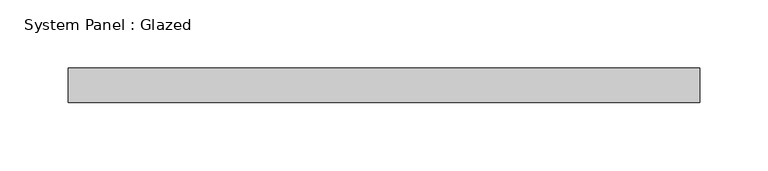
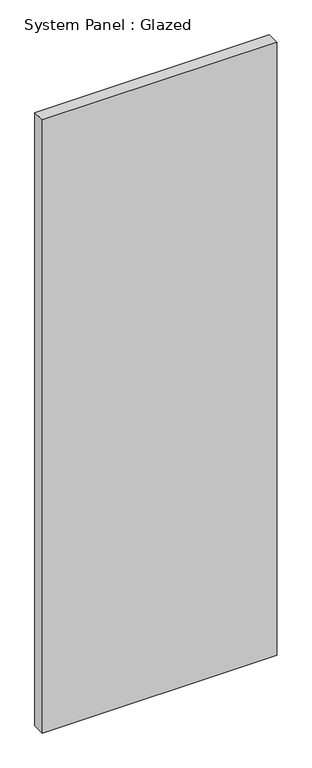
"""IFC4 building model written with IfcOpenShell, lengths in millimetres: plate geometry, System Panel : Glazed."""

from ifc_helpers import new_model, si_unit, origin, origin_with_axes, place, context, project, spatial, polyline, outline, extrude, source, transform, mapped, element, save


def system_panel_glazed_83e43f9b(model_context):
    return source(origin(), model_context, "Body", "SweptSolid", [
        extrude(outline(polyline([(231.775, 19.05), (-231.775, 19.05), (-231.775, 44.45), (231.775, 44.45), (231.775, 19.05)])), origin_with_axes(), (0.0, 0.0, 1.0), 1281.187673),
    ])


if __name__ == "__main__":
    model = new_model("IFC4")
    model_context = context("Model", 3, world=origin())
    ifc_project = project(units=[si_unit("LENGTHUNIT", "METRE", prefix="MILLI")], contexts=[model_context])
    site = spatial("IfcSite", under=ifc_project)
    building = spatial("IfcBuilding", under=site)
    placement = place(None, origin())
    system_panel_glazed_shape = system_panel_glazed_83e43f9b(model_context)
    element("IfcPlate", 1, ObjectType="System Panel : Glazed", at=placement, inside=building, context=model_context, shape_type="MappedRepresentation", body=[
        mapped(system_panel_glazed_shape, transform((0.0, 0.0, 0.0), x_axis=(1.0, 0.0, 0.0), y_axis=(0.0, 1.0, 0.0), z_axis=(0.0, 0.0, 1.0))),
    ])
    save(model, "model.ifc")

# Revit data of these elements
# Type "System Panel : Glazed"
#   Construction Type Id = "GSP4R"
#   Analytic Construction = "1/8 in Pilkington single glazing"
#   Visual Light Transmittance = 0.9
#   Solar Heat Gain Coefficient = 0.86
#   Heat Transfer Coefficient (U) = 1.18115 BTU/(h·ft²·°F)
#   Define Thermal Properties by = 1
# Element 1 (IfcPlate, "System Panel : Glazed")
#   Materials on its faces: "Glass"
# Materials
#   "Glass": class "Glass", colour RGB 0 128 192, transparency 0.75, Description = "Soda Lime Glass", Cost = 0
